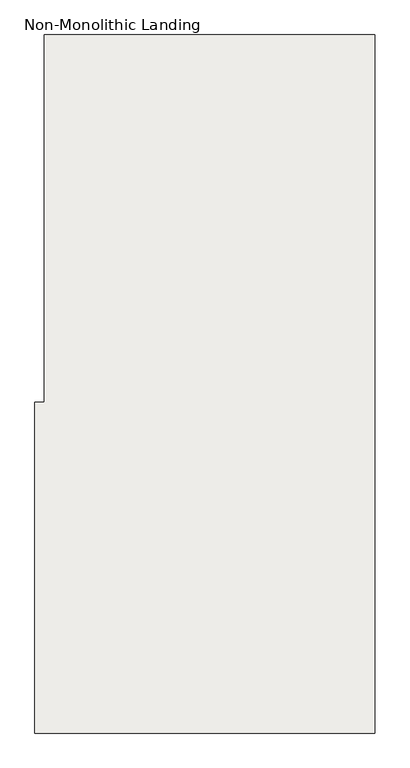
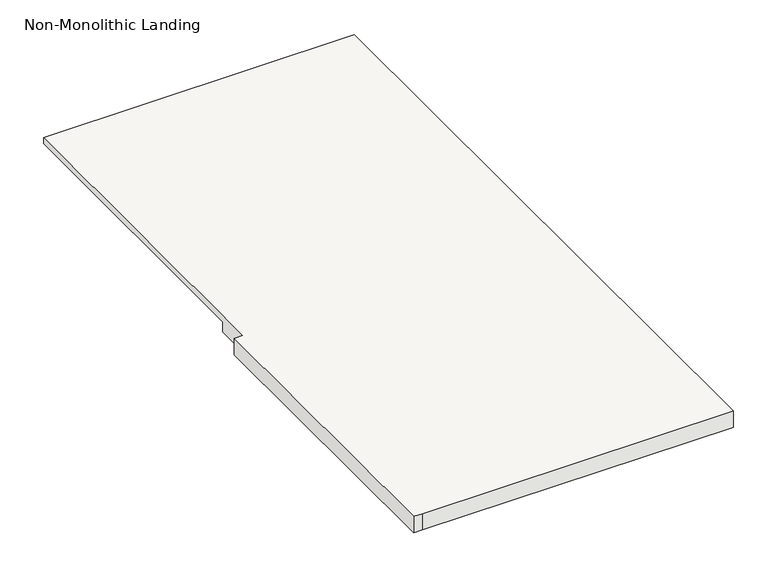
"""IFC4 building model written with IfcOpenShell, lengths in millimetres: slab geometry, Non-Monolithic Landing."""

from ifc_helpers import new_model, si_unit, origin, place, context, project, spatial, faceted_brep, source, transform, mapped, element, save


def non_monolithic_landing_9a06da9a(model_context):
    return source(origin(), model_context, "Body", "Brep", [
        faceted_brep([(923.4845537, -3822.9544725, 27184.35), (948.8845537, -3822.9544725, 27158.95), (948.8845537, -4737.3544725, 27158.95), (923.4845537, -4737.3544725, 27184.35), (923.4845537, -4838.9544725, 27203.4), (898.0845537, -4838.9544725, 27203.4), (898.0845537, -5753.3544725, 27203.4), (923.4845537, -5753.3544725, 27203.4), (1837.8845537, -5753.3544725, 27203.4), (1837.8845537, -3822.9544725, 27203.4), (923.4845537, -3822.9544725, 27203.4), (948.8845537, -4737.3544725, 27152.6), (948.8845537, -3822.9544725, 27152.6), (1837.8845537, -3822.9544725, 27152.6), (1837.8845537, -5753.3544725, 27152.6), (923.4845537, -5753.3544725, 27152.6), (898.0845537, -5753.3544725, 27152.6), (898.0845537, -4838.9544725, 27152.6), (923.4845537, -4838.9544725, 27152.6), (923.4845537, -4737.3544725, 27152.6)], [[[0, 1, 2, 3]], [[4, 5, 6, 7, 8, 9, 10]], [[11, 12, 13, 14, 15, 16, 17, 18, 19]], [[12, 11, 2, 1]], [[11, 19, 3, 2]], [[4, 10, 0, 3, 19, 18]], [[5, 4, 18, 17]], [[6, 5, 17, 16]], [[7, 6, 16, 15]], [[8, 7, 15, 14]], [[9, 8, 14, 13]], [[10, 9, 13, 12, 1, 0]]]),
    ])


if __name__ == "__main__":
    model = new_model("IFC4")
    model_context = context("Model", 3, world=origin())
    ifc_project = project(units=[si_unit("LENGTHUNIT", "METRE", prefix="MILLI")], contexts=[model_context])
    site = spatial("IfcSite", under=ifc_project)
    building = spatial("IfcBuilding", under=site)
    placement = place(None, origin())
    non_monolithic_landing_shape = non_monolithic_landing_9a06da9a(model_context)
    element("IfcSlab", 1, ObjectType="Non-Monolithic Landing", at=placement, inside=building, context=model_context, shape_type="MappedRepresentation", body=[
        mapped(non_monolithic_landing_shape, transform((0.0, 0.0, 0.0), x_axis=(1.0, 0.0, 0.0), y_axis=(0.0, 1.0, 0.0), z_axis=(0.0, 0.0, 1.0))),
    ])
    save(model, "model.ifc")
